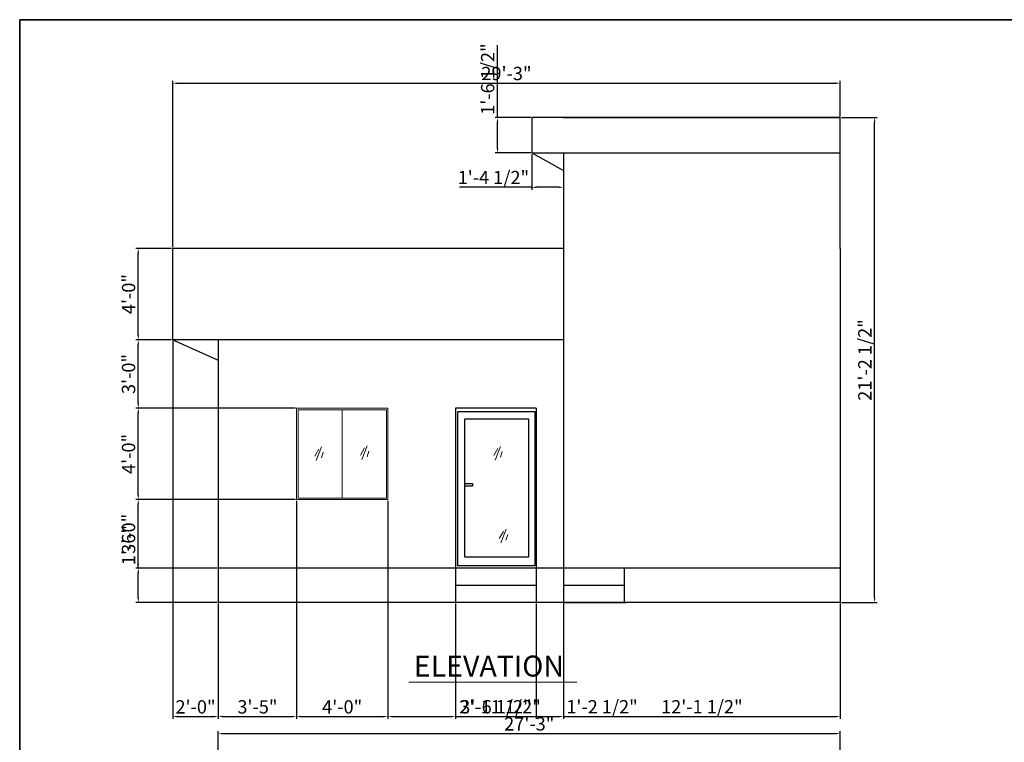
# Model space of a CAD drawing. Units: inches. Extents: x 1863 to 2938, y 1238 to 2492.
# Tile 10 of 12: x 1863 to 2381, y 2112 to 2492. Entities that reach past the tile are written whole.
import ezdxf

# ---------------------------------------------------------------- set-up
doc = ezdxf.new("R2010")
doc.units = ezdxf.units.IN
for name, color, linetype, lineweight in [('A-ANNO-DIMS', 2, 'Continuous', 18), ('A-ANNO-TEXT', 7, 'Continuous', 18), ('A-ANNO-TTLB', 7, 'Continuous', 35), ('A-DOOR', 3, 'Continuous', 25), ('A-ELEV', 7, 'Continuous', 25), ('A-GLAZ', 4, 'Continuous', 18)]:
    doc.layers.add(name, color=color, linetype=linetype, lineweight=lineweight)
doc.styles.get("Standard").update_dxf_attribs({"font": 'arial.ttf'})
doc.dimstyles.new('ISO-25', dxfattribs={"dimtxt": 7, "dimasz": 2.5, "dimexe": 1.25, "dimexo": 0.625, "dimtad": 1, "dimdec": 0, "dimlunit": 3, "dimtxsty": 'Standard', "dimcen": 2.5, "dimadec": 0, "dimazin": 0, "dimtfac": 1, "dimtdec": 0, "dimtmove": 0, "dimatfit": 3, "dimfxl": 1, "dimarcsym": 0})

# ---------------------------------------------------------------- blocks, each defined once
blk = doc.blocks.new('*D2')
at = {"layer": 'A-ANNO-DIMS', "color": 0, "lineweight": -2, "transparency": 16777216}
for p, q in [((1967.64, 2077.19), (1967.64, 2118.26)), ((2294.64, 2077.19), (2294.64, 2118.26)), ((1970.14, 2117.01), (2292.14, 2117.01))]:
    blk.add_line(p, q, dxfattribs=at)
at = {"layer": 'A-ANNO-DIMS', "color": 0, "transparency": 16777216}
for points in [[(1970.14, 2117.43), (1970.14, 2116.59), (1967.64, 2117.01)], [(2292.14, 2117.43), (2292.14, 2116.59), (2294.64, 2117.01)]]:
    blk.add_solid(points, dxfattribs=at)
at = {"layer": 'Defpoints', "color": 0, "transparency": 16777216}
for p in [(2294.64, 2117.01), (1967.64, 2076.56), (2294.64, 2076.56)]:
    blk.add_point(p, dxfattribs=at)
at = {"layer": 'A-ANNO-DIMS', "color": 0, "transparency": 16777216, "insert": (2131.14, 2121.21), "char_height": 7, "attachment_point": 5}
blk.add_mtext('27\'-3"', dxfattribs=at)
blk = doc.blocks.new('GLASS-REFLECTION')
for p, q in [((2.24, 6.11), (0, 2.35)), ((3.64, 7.18), (0.84, 0)), ((4.51, 4.47), (3.5, 1.46))]:
    blk.add_line(p, q)
blk = doc.blocks.new('*D71')
at = {"layer": 'A-ANNO-DIMS', "color": 0, "lineweight": -2, "transparency": 16777216}
for p, q in [((1943.64, 2372.62), (1943.64, 2460.06)), ((2294.64, 2441.34), (2294.64, 2460.06)), ((1946.14, 2458.81), (2292.14, 2458.81))]:
    blk.add_line(p, q, dxfattribs=at)
at = {"layer": 'A-ANNO-DIMS', "color": 0, "transparency": 16777216}
for points in [[(1946.14, 2459.23), (1946.14, 2458.4), (1943.64, 2458.81)], [(2292.14, 2459.23), (2292.14, 2458.4), (2294.64, 2458.81)]]:
    blk.add_solid(points, dxfattribs=at)
at = {"layer": 'Defpoints', "color": 0, "transparency": 16777216}
for p in [(2294.64, 2458.81), (2294.64, 2440.71), (1943.64, 2371.99)]:
    blk.add_point(p, dxfattribs=at)
at = {"layer": 'A-ANNO-DIMS', "color": 0, "transparency": 16777216, "insert": (2119.14, 2463.01), "char_height": 7, "attachment_point": 5}
blk.add_mtext('29\'-3"', dxfattribs=at)
blk = doc.blocks.new('*D72')
at = {"layer": 'A-ANNO-DIMS', "color": 0, "lineweight": -2, "transparency": 16777216}
for p, q in [((2295.26, 2440.71), (2313.99, 2440.71)), ((2312.74, 2188.49), (2312.74, 2438.21)), ((2295.26, 2185.99), (2313.99, 2185.99))]:
    blk.add_line(p, q, dxfattribs=at)
at = {"layer": 'A-ANNO-DIMS', "color": 0, "transparency": 16777216}
for points in [[(2312.32, 2438.21), (2313.16, 2438.21), (2312.74, 2440.71)], [(2312.32, 2188.49), (2313.16, 2188.49), (2312.74, 2185.99)]]:
    blk.add_solid(points, dxfattribs=at)
at = {"layer": 'Defpoints', "color": 0, "transparency": 16777216}
for p in [(2294.64, 2440.71), (2312.74, 2440.71), (2294.64, 2185.99)]:
    blk.add_point(p, dxfattribs=at)
at = {"layer": 'A-ANNO-DIMS', "color": 0, "transparency": 16777216, "insert": (2308.5, 2313.35), "char_height": 7, "attachment_point": 5, "rotation": 90}
blk.add_mtext('21\'-2 1/2"', dxfattribs=at)
blk = doc.blocks.new('*D73')
at = {"layer": 'A-ANNO-DIMS', "color": 0, "lineweight": -2, "transparency": 16777216}
for p, q in [((2114.42, 2440.71), (2114.42, 2478.72)), ((2131.9, 2440.71), (2113.17, 2440.71)), ((2114.42, 2424.71), (2114.42, 2438.21)), ((2131.9, 2422.21), (2113.17, 2422.21))]:
    blk.add_line(p, q, dxfattribs=at)
at = {"layer": 'A-ANNO-DIMS', "color": 0, "transparency": 16777216}
for points in [[(2114.01, 2438.21), (2114.84, 2438.21), (2114.42, 2440.71)], [(2114.01, 2424.71), (2114.84, 2424.71), (2114.42, 2422.21)]]:
    blk.add_solid(points, dxfattribs=at)
at = {"layer": 'Defpoints', "color": 0, "transparency": 16777216}
for p in [(2114.42, 2440.71), (2132.52, 2440.71), (2132.52, 2422.21)]:
    blk.add_point(p, dxfattribs=at)
at = {"layer": 'A-ANNO-DIMS', "color": 0, "transparency": 16777216, "insert": (2110.18, 2460.97), "char_height": 7, "attachment_point": 5, "rotation": 90}
blk.add_mtext('1\'-6 1/2"', dxfattribs=at)
blk = doc.blocks.new('*D74')
at = {"layer": 'A-ANNO-DIMS', "color": 0, "lineweight": -2, "transparency": 16777216}
for p, q in [((2132.52, 2421.58), (2132.52, 2402.86)), ((2149.14, 2421.58), (2149.14, 2402.86)), ((2132.52, 2404.11), (2094.51, 2404.11)), ((2146.64, 2404.11), (2135.02, 2404.11))]:
    blk.add_line(p, q, dxfattribs=at)
at = {"layer": 'A-ANNO-DIMS', "color": 0, "transparency": 16777216}
for points in [[(2135.02, 2404.52), (2135.02, 2403.69), (2132.52, 2404.11)], [(2146.64, 2404.52), (2146.64, 2403.69), (2149.14, 2404.11)]]:
    blk.add_solid(points, dxfattribs=at)
at = {"layer": 'Defpoints', "color": 0, "transparency": 16777216}
for p in [(2132.52, 2422.21), (2149.14, 2422.21), (2132.52, 2404.11)]:
    blk.add_point(p, dxfattribs=at)
at = {"layer": 'A-ANNO-DIMS', "color": 0, "transparency": 16777216, "insert": (2112.27, 2408.35), "char_height": 7, "attachment_point": 5}
blk.add_mtext('1\'-4 1/2"', dxfattribs=at)
blk = doc.blocks.new('*D75')
at = {"layer": 'A-ANNO-DIMS', "color": 0, "lineweight": -2, "transparency": 16777216}
for p, q in [((1943.01, 2371.99), (1924.29, 2371.99)), ((1925.54, 2326.49), (1925.54, 2369.49)), ((1943.01, 2323.99), (1924.29, 2323.99))]:
    blk.add_line(p, q, dxfattribs=at)
at = {"layer": 'A-ANNO-DIMS', "color": 0, "transparency": 16777216}
for points in [[(1925.12, 2369.49), (1925.96, 2369.49), (1925.54, 2371.99)], [(1925.12, 2326.49), (1925.96, 2326.49), (1925.54, 2323.99)]]:
    blk.add_solid(points, dxfattribs=at)
at = {"layer": 'Defpoints', "color": 0, "transparency": 16777216}
for p in [(1925.54, 2371.99), (1943.64, 2371.99), (1943.64, 2323.99)]:
    blk.add_point(p, dxfattribs=at)
at = {"layer": 'A-ANNO-DIMS', "color": 0, "transparency": 16777216, "insert": (1921.34, 2347.99), "char_height": 7, "attachment_point": 5, "rotation": 90}
blk.add_mtext('4\'-0"', dxfattribs=at)
blk = doc.blocks.new('*D76')
at = {"layer": 'A-ANNO-DIMS', "color": 0, "lineweight": -2, "transparency": 16777216}
for p, q in [((1925.54, 2203.99), (1925.54, 2225.69)), ((1967.01, 2203.99), (1924.29, 2203.99)), ((1925.54, 2188.49), (1925.54, 2201.49)), ((1967.01, 2185.99), (1924.29, 2185.99))]:
    blk.add_line(p, q, dxfattribs=at)
at = {"layer": 'A-ANNO-DIMS', "color": 0, "transparency": 16777216}
for points in [[(1925.12, 2201.49), (1925.96, 2201.49), (1925.54, 2203.99)], [(1925.12, 2188.49), (1925.96, 2188.49), (1925.54, 2185.99)]]:
    blk.add_solid(points, dxfattribs=at)
at = {"layer": 'Defpoints', "color": 0, "transparency": 16777216}
for p in [(1925.54, 2203.99), (1967.64, 2203.99), (1967.64, 2185.99)]:
    blk.add_point(p, dxfattribs=at)
at = {"layer": 'A-ANNO-DIMS', "color": 0, "transparency": 16777216, "insert": (1921.34, 2216.09), "char_height": 7, "attachment_point": 5, "rotation": 90}
blk.add_mtext('1\'-6"', dxfattribs=at)
blk = doc.blocks.new('*D77')
at = {"layer": 'A-ANNO-DIMS', "color": 0, "lineweight": -2, "transparency": 16777216}
for p, q in [((1943.64, 2323.37), (1943.64, 2124.7)), ((1967.64, 2185.37), (1967.64, 2124.7)), ((1946.14, 2125.95), (1965.14, 2125.95))]:
    blk.add_line(p, q, dxfattribs=at)
at = {"layer": 'A-ANNO-DIMS', "color": 0, "transparency": 16777216}
for points in [[(1946.14, 2126.37), (1946.14, 2125.54), (1943.64, 2125.95)], [(1965.14, 2126.37), (1965.14, 2125.54), (1967.64, 2125.95)]]:
    blk.add_solid(points, dxfattribs=at)
at = {"layer": 'Defpoints', "color": 0, "transparency": 16777216}
for p in [(1943.64, 2323.99), (1967.64, 2185.99), (1967.64, 2125.95)]:
    blk.add_point(p, dxfattribs=at)
at = {"layer": 'A-ANNO-DIMS', "color": 0, "transparency": 16777216, "insert": (1955.64, 2130.15), "char_height": 7, "attachment_point": 5}
blk.add_mtext('2\'-0"', dxfattribs=at)
blk = doc.blocks.new('*D78')
at = {"layer": 'A-ANNO-DIMS', "color": 0, "lineweight": -2, "transparency": 16777216}
for p, q in [((2008.76, 2239.37), (2008.76, 2124.7)), ((1967.64, 2185.37), (1967.64, 2124.7)), ((1970.14, 2125.95), (2006.26, 2125.95))]:
    blk.add_line(p, q, dxfattribs=at)
at = {"layer": 'A-ANNO-DIMS', "color": 0, "transparency": 16777216}
for points in [[(1970.14, 2126.37), (1970.14, 2125.54), (1967.64, 2125.95)], [(2006.26, 2126.37), (2006.26, 2125.54), (2008.76, 2125.95)]]:
    blk.add_solid(points, dxfattribs=at)
at = {"layer": 'Defpoints', "color": 0, "transparency": 16777216}
for p in [(2008.76, 2239.99), (1967.64, 2185.99), (2008.76, 2125.95)]:
    blk.add_point(p, dxfattribs=at)
at = {"layer": 'A-ANNO-DIMS', "color": 0, "transparency": 16777216, "insert": (1988.2, 2130.16), "char_height": 7, "attachment_point": 5}
blk.add_mtext('3\'-5"', dxfattribs=at)
blk = doc.blocks.new('*D79')
at = {"layer": 'A-ANNO-DIMS', "color": 0, "lineweight": -2, "transparency": 16777216}
for p, q in [((2008.76, 2239.37), (2008.76, 2124.7)), ((2056.76, 2239.37), (2056.76, 2124.7)), ((2011.26, 2125.95), (2054.26, 2125.95))]:
    blk.add_line(p, q, dxfattribs=at)
at = {"layer": 'A-ANNO-DIMS', "color": 0, "transparency": 16777216}
for points in [[(2011.26, 2126.37), (2011.26, 2125.54), (2008.76, 2125.95)], [(2054.26, 2126.37), (2054.26, 2125.54), (2056.76, 2125.95)]]:
    blk.add_solid(points, dxfattribs=at)
at = {"layer": 'Defpoints', "color": 0, "transparency": 16777216}
for p in [(2008.76, 2239.99), (2056.76, 2239.99), (2056.76, 2125.95)]:
    blk.add_point(p, dxfattribs=at)
at = {"layer": 'A-ANNO-DIMS', "color": 0, "transparency": 16777216, "insert": (2032.76, 2130.15), "char_height": 7, "attachment_point": 5}
blk.add_mtext('4\'-0"', dxfattribs=at)
blk = doc.blocks.new('*D80')
at = {"layer": 'A-ANNO-DIMS', "color": 0, "lineweight": -2, "transparency": 16777216}
for p, q in [((2056.76, 2239.37), (2056.76, 2124.7)), ((2092.4, 2185.37), (2092.4, 2124.7)), ((2059.26, 2125.95), (2089.9, 2125.95)), ((2092.4, 2125.95), (2136.63, 2125.95))]:
    blk.add_line(p, q, dxfattribs=at)
at = {"layer": 'A-ANNO-DIMS', "color": 0, "transparency": 16777216}
for points in [[(2059.26, 2126.37), (2059.26, 2125.54), (2056.76, 2125.95)], [(2089.9, 2126.37), (2089.9, 2125.54), (2092.4, 2125.95)]]:
    blk.add_solid(points, dxfattribs=at)
at = {"layer": 'Defpoints', "color": 0, "transparency": 16777216}
for p in [(2056.76, 2239.99), (2092.4, 2185.99), (2092.4, 2125.95)]:
    blk.add_point(p, dxfattribs=at)
at = {"layer": 'A-ANNO-DIMS', "color": 0, "transparency": 16777216, "insert": (2115.77, 2130.2), "char_height": 7, "attachment_point": 5}
blk.add_mtext('2\'-11 1/2"', dxfattribs=at)
blk = doc.blocks.new('*D81')
at = {"layer": 'A-ANNO-DIMS', "color": 0, "lineweight": -2, "transparency": 16777216}
for p, q in [((2092.4, 2185.37), (2092.4, 2124.7)), ((2134.81, 2185.37), (2134.81, 2124.7)), ((2094.9, 2125.95), (2132.31, 2125.95))]:
    blk.add_line(p, q, dxfattribs=at)
at = {"layer": 'A-ANNO-DIMS', "color": 0, "transparency": 16777216}
for points in [[(2094.9, 2126.37), (2094.9, 2125.54), (2092.4, 2125.95)], [(2132.31, 2126.37), (2132.31, 2125.54), (2134.81, 2125.95)]]:
    blk.add_solid(points, dxfattribs=at)
at = {"layer": 'Defpoints', "color": 0, "transparency": 16777216}
for p in [(2092.4, 2185.99), (2134.81, 2185.99), (2134.81, 2125.95)]:
    blk.add_point(p, dxfattribs=at)
at = {"layer": 'A-ANNO-DIMS', "color": 0, "transparency": 16777216, "insert": (2113.61, 2130.2), "char_height": 7, "attachment_point": 5}
blk.add_mtext('3\'-6 1/2"', dxfattribs=at)
blk = doc.blocks.new('*D82')
at = {"layer": 'A-ANNO-DIMS', "color": 0, "lineweight": -2, "transparency": 16777216}
for p, q in [((2134.81, 2185.37), (2134.81, 2124.7)), ((2149.14, 2185.37), (2149.14, 2124.7)), ((2137.31, 2125.95), (2146.64, 2125.95)), ((2149.14, 2125.95), (2187.15, 2125.95))]:
    blk.add_line(p, q, dxfattribs=at)
at = {"layer": 'A-ANNO-DIMS', "color": 0, "transparency": 16777216}
for points in [[(2137.31, 2126.37), (2137.31, 2125.54), (2134.81, 2125.95)], [(2146.64, 2126.37), (2146.64, 2125.54), (2149.14, 2125.95)]]:
    blk.add_solid(points, dxfattribs=at)
at = {"layer": 'Defpoints', "color": 0, "transparency": 16777216}
for p in [(2134.81, 2185.99), (2149.14, 2185.99), (2149.14, 2125.95)]:
    blk.add_point(p, dxfattribs=at)
at = {"layer": 'A-ANNO-DIMS', "color": 0, "transparency": 16777216, "insert": (2169.39, 2130.2), "char_height": 7, "attachment_point": 5}
blk.add_mtext('1\'-2 1/2"', dxfattribs=at)
blk = doc.blocks.new('*D83')
at = {"layer": 'A-ANNO-DIMS', "color": 0, "lineweight": -2, "transparency": 16777216}
for p, q in [((2149.14, 2185.37), (2149.14, 2124.7)), ((2294.64, 2185.37), (2294.64, 2124.7)), ((2151.64, 2125.95), (2292.14, 2125.95))]:
    blk.add_line(p, q, dxfattribs=at)
at = {"layer": 'A-ANNO-DIMS', "color": 0, "transparency": 16777216}
for points in [[(2151.64, 2126.37), (2151.64, 2125.54), (2149.14, 2125.95)], [(2292.14, 2126.37), (2292.14, 2125.54), (2294.64, 2125.95)]]:
    blk.add_solid(points, dxfattribs=at)
at = {"layer": 'Defpoints', "color": 0, "transparency": 16777216}
for p in [(2149.14, 2185.99), (2294.64, 2185.99), (2294.64, 2125.95)]:
    blk.add_point(p, dxfattribs=at)
at = {"layer": 'A-ANNO-DIMS', "color": 0, "transparency": 16777216, "insert": (2221.89, 2130.2), "char_height": 7, "attachment_point": 5}
blk.add_mtext('12\'-1 1/2"', dxfattribs=at)
blk = doc.blocks.new('*D84')
at = {"layer": 'A-ANNO-DIMS', "color": 0, "lineweight": -2, "transparency": 16777216}
for p, q in [((2008.14, 2287.99), (1924.29, 2287.99)), ((1925.54, 2242.49), (1925.54, 2285.49)), ((2008.14, 2239.99), (1924.29, 2239.99))]:
    blk.add_line(p, q, dxfattribs=at)
at = {"layer": 'A-ANNO-DIMS', "color": 0, "transparency": 16777216}
for points in [[(1925.12, 2285.49), (1925.96, 2285.49), (1925.54, 2287.99)], [(1925.12, 2242.49), (1925.96, 2242.49), (1925.54, 2239.99)]]:
    blk.add_solid(points, dxfattribs=at)
at = {"layer": 'Defpoints', "color": 0, "transparency": 16777216}
for p in [(1925.54, 2287.99), (2008.76, 2287.99), (2008.76, 2239.99)]:
    blk.add_point(p, dxfattribs=at)
at = {"layer": 'A-ANNO-DIMS', "color": 0, "transparency": 16777216, "insert": (1921.34, 2263.99), "char_height": 7, "attachment_point": 5, "rotation": 90}
blk.add_mtext('4\'-0"', dxfattribs=at)
blk = doc.blocks.new('*D85')
at = {"layer": 'A-ANNO-DIMS', "color": 0, "lineweight": -2, "transparency": 16777216}
for p, q in [((2008.14, 2239.99), (1924.29, 2239.99)), ((1925.54, 2206.49), (1925.54, 2237.49)), ((1967.01, 2203.99), (1924.29, 2203.99))]:
    blk.add_line(p, q, dxfattribs=at)
at = {"layer": 'A-ANNO-DIMS', "color": 0, "transparency": 16777216}
for points in [[(1925.12, 2237.49), (1925.96, 2237.49), (1925.54, 2239.99)], [(1925.12, 2206.49), (1925.96, 2206.49), (1925.54, 2203.99)]]:
    blk.add_solid(points, dxfattribs=at)
at = {"layer": 'Defpoints', "color": 0, "transparency": 16777216}
for p in [(1925.54, 2239.99), (2008.76, 2239.99), (1967.64, 2203.99)]:
    blk.add_point(p, dxfattribs=at)
at = {"layer": 'A-ANNO-DIMS', "color": 0, "transparency": 16777216, "insert": (1921.34, 2221.99), "char_height": 7, "attachment_point": 5, "rotation": 90}
blk.add_mtext('3\'-0"', dxfattribs=at)
blk = doc.blocks.new('*D86')
at = {"layer": 'A-ANNO-DIMS', "color": 0, "lineweight": -2, "transparency": 16777216}
for p, q in [((1943.01, 2323.99), (1924.29, 2323.99)), ((1925.54, 2290.49), (1925.54, 2321.49)), ((2008.14, 2287.99), (1924.29, 2287.99))]:
    blk.add_line(p, q, dxfattribs=at)
at = {"layer": 'A-ANNO-DIMS', "color": 0, "transparency": 16777216}
for points in [[(1925.12, 2321.49), (1925.96, 2321.49), (1925.54, 2323.99)], [(1925.12, 2290.49), (1925.96, 2290.49), (1925.54, 2287.99)]]:
    blk.add_solid(points, dxfattribs=at)
at = {"layer": 'Defpoints', "color": 0, "transparency": 16777216}
for p in [(1925.54, 2323.99), (1943.64, 2323.99), (2008.76, 2287.99)]:
    blk.add_point(p, dxfattribs=at)
at = {"layer": 'A-ANNO-DIMS', "color": 0, "transparency": 16777216, "insert": (1921.34, 2305.99), "char_height": 7, "attachment_point": 5, "rotation": 90}
blk.add_mtext('3\'-0"', dxfattribs=at)

msp = doc.modelspace()

# ---------------------------------------------------------------- linework, layer by layer
at = {"layer": 'A-ANNO-TEXT'}
msp.add_line((2067.73, 2144.05), (2156.2, 2144.05), dxfattribs=at)
at = {"layer": 'A-ANNO-TTLB'}
msp.add_lwpolyline([(1863.2, 2492.19), (2938.41, 2492.19), (2938.41, 1253.47), (1863.2, 1253.47)], close=True, dxfattribs=at)
at = {"layer": 'A-DOOR'}
for p, q in [((2092.4, 2287.99), (2092.4, 2203.99)), ((2134.81, 2287.99), (2092.4, 2287.99)), ((2134.81, 2287.99), (2134.81, 2203.99))]:
    msp.add_line(p, q, dxfattribs=at)
for points in [[(2093.53, 2286.35), (2134.13, 2286.35), (2134.13, 2205.1), (2093.53, 2205.1)], [(2097.2, 2282.38), (2130.66, 2282.38), (2130.66, 2209.66), (2097.2, 2209.66)], [(2097.2, 2248.49), (2101.34, 2248.49), (2101.34, 2246.99), (2097.2, 2246.99)]]:
    msp.add_lwpolyline(points, close=True, dxfattribs=at)
at = {"layer": 'A-ELEV'}
for p, q in [((2149.14, 2440.71), (2132.52, 2440.71)), ((2132.52, 2440.71), (2132.52, 2422.21)), ((2149.14, 2440.71), (2294.64, 2440.71)), ((2294.64, 2440.71), (2149.14, 2440.71)), ((2294.64, 2371.99), (2294.64, 2440.71)), ((2132.52, 2422.21), (2149.14, 2422.21)), ((2132.52, 2422.21), (2149.14, 2412.88)), ((2149.14, 2422.21), (2149.14, 2203.99)), ((2149.14, 2422.21), (2294.64, 2422.21)), ((2149.14, 2371.99), (1943.64, 2371.99)), ((1943.64, 2323.99), (1943.64, 2371.99)), ((2294.64, 2371.99), (2294.64, 2185.99)), ((2149.14, 2323.99), (1943.64, 2323.99)), ((1943.64, 2323.99), (1967.64, 2313.19)), ((1967.64, 2323.99), (1967.64, 2185.99)), ((2294.64, 2203.99), (1967.64, 2203.99)), ((2092.4, 2203.99), (2092.4, 2185.99)), ((2134.81, 2203.99), (2134.81, 2185.99)), ((2149.14, 2203.99), (2149.14, 2185.99)), ((2181.02, 2203.99), (2181.02, 2185.99)), ((2092.4, 2194.99), (2134.81, 2194.99)), ((2149.14, 2194.99), (2181.02, 2194.99)), ((2294.64, 2185.99), (1967.64, 2185.99)), ((2149.14, 2185.99), (2181.89, 2185.99))]:
    msp.add_line(p, q, dxfattribs=at)
at = {"layer": 'A-GLAZ'}
for p, q in [((2008.76, 2287.99), (2008.76, 2239.99)), ((2056.76, 2287.99), (2008.76, 2287.99)), ((2032.78, 2287.16), (2032.78, 2240.8)), ((2056.76, 2287.99), (2056.76, 2239.99)), ((2056.76, 2239.99), (2008.76, 2239.99))]:
    msp.add_line(p, q, dxfattribs=at)
msp.add_lwpolyline([(2009.55, 2287.16), (2056.01, 2287.16), (2056.01, 2240.8), (2009.55, 2240.8)], close=True, dxfattribs=at)

# ---------------------------------------------------------------- block references
for p in [(2018.31, 2260.45), (2042.34, 2261.02), (2112.45, 2260.74), (2115.34, 2217.19)]:
    msp.add_blockref('GLASS-REFLECTION', p, dxfattribs=at)

# ---------------------------------------------------------------- texts
at = {"layer": 'A-ANNO-TEXT', "insert": (2070.47, 2157.99), "char_height": 11, "attachment_point": 1}
msp.add_mtext_dynamic_manual_height_columns('ELEVATION', width=259.8904, gutter_width=12.5, heights=[0], dxfattribs=at)

# ---------------------------------------------------------------- dimensions: what is measured, and where the dimension line sits
at = {"layer": 'A-ANNO-DIMS'}
for base, p1, p2, angle, picture, middle in [((2114.42, 2440.71), (2132.52, 2422.21), (2132.52, 2440.71), 90, '*D73', (2110.18, 2460.97)), ((2312.74, 2440.71), (2294.64, 2185.99), (2294.64, 2440.71), 90, '*D72', (2308.5, 2313.35)), ((2132.52, 2404.11), (2149.14, 2422.21), (2132.52, 2422.21), 180, '*D74', (2112.27, 2408.35)), ((1925.54, 2371.99), (1943.64, 2323.99), (1943.64, 2371.99), 90, '*D75', (1921.34, 2347.99)), ((1925.54, 2323.99), (2008.76, 2287.99), (1943.64, 2323.99), 90, '*D86', (1921.34, 2305.99)), ((1925.54, 2287.99), (2008.76, 2239.99), (2008.76, 2287.99), 90, '*D84', (1921.34, 2263.99)), ((1925.54, 2239.99), (1967.64, 2203.99), (2008.76, 2239.99), 90, '*D85', (1921.34, 2221.99)), ((1925.54, 2203.99), (1967.64, 2185.99), (1967.64, 2203.99), 90, '*D76', (1921.34, 2216.09))]:
    dim = msp.add_linear_dim(base=base, p1=p1, p2=p2, angle=angle, dimstyle='ISO-25', override={"dimdec": 1, "dimlfac": 1, "dimrnd": 0, "dimzin": 1, "dimdsep": 46, "dimlunit": 4, "dimfrac": 2}, dxfattribs=at)
    dim.commit()
    dim.dimension.update_dxf_attribs({"geometry": picture, "text_midpoint": middle})
for base, p1, p2, override, picture, middle in [((2294.64, 2458.81), (1943.64, 2371.99), (2294.64, 2440.71), {"dimdec": 1, "dimlfac": 1, "dimrnd": 0, "dimzin": 1, "dimdsep": 46, "dimlunit": 4, "dimfrac": 2}, '*D71', (2119.14, 2463.01)), ((1967.64, 2125.95), (1943.64, 2323.99), (1967.64, 2185.99), {"dimdec": 1, "dimlfac": 1, "dimrnd": 0, "dimzin": 1, "dimdsep": 46, "dimlunit": 4, "dimfrac": 2}, '*D77', (1955.64, 2130.15)), ((2008.76, 2125.95), (1967.64, 2185.99), (2008.76, 2239.99), {"dimdec": 1, "dimlfac": 1, "dimrnd": 0, "dimzin": 1, "dimdsep": 46, "dimlunit": 4, "dimfrac": 2}, '*D78', (1988.2, 2130.16)), ((2056.76, 2125.95), (2008.76, 2239.99), (2056.76, 2239.99), {"dimdec": 1, "dimlfac": 1, "dimrnd": 0, "dimzin": 1, "dimdsep": 46, "dimlunit": 4, "dimfrac": 2}, '*D79', (2032.76, 2130.15)), ((2092.4, 2125.95), (2056.76, 2239.99), (2092.4, 2185.99), {"dimdec": 1, "dimlfac": 1, "dimrnd": 0, "dimzin": 1, "dimdsep": 46, "dimlunit": 4, "dimfrac": 2}, '*D80', (2115.77, 2130.2)), ((2134.81, 2125.95), (2092.4, 2185.99), (2134.81, 2185.99), {"dimdec": 1, "dimlfac": 1, "dimrnd": 0, "dimzin": 1, "dimdsep": 46, "dimlunit": 4, "dimfrac": 2}, '*D81', (2113.61, 2130.2)), ((2149.14, 2125.95), (2134.81, 2185.99), (2149.14, 2185.99), {"dimdec": 1, "dimlfac": 1, "dimrnd": 0, "dimzin": 1, "dimdsep": 46, "dimlunit": 4, "dimfrac": 2}, '*D82', (2169.39, 2130.2)), ((2294.64, 2125.95), (2149.14, 2185.99), (2294.64, 2185.99), {"dimdec": 1, "dimlfac": 1, "dimrnd": 0, "dimzin": 1, "dimdsep": 46, "dimlunit": 4, "dimfrac": 2}, '*D83', (2221.89, 2130.2)), ((2294.64, 2117.01), (1967.64, 2076.56), (2294.64, 2076.56), {"dimclrd": 0, "dimclre": 0, "dimclrt": 0}, '*D2', (2131.14, 2121.21))]:
    dim = msp.add_linear_dim(base=base, p1=p1, p2=p2, dimstyle='ISO-25', override=override, dxfattribs=at)
    dim.commit()
    dim.dimension.update_dxf_attribs({"geometry": picture, "text_midpoint": middle})

doc.saveas('drawing.dxf')
